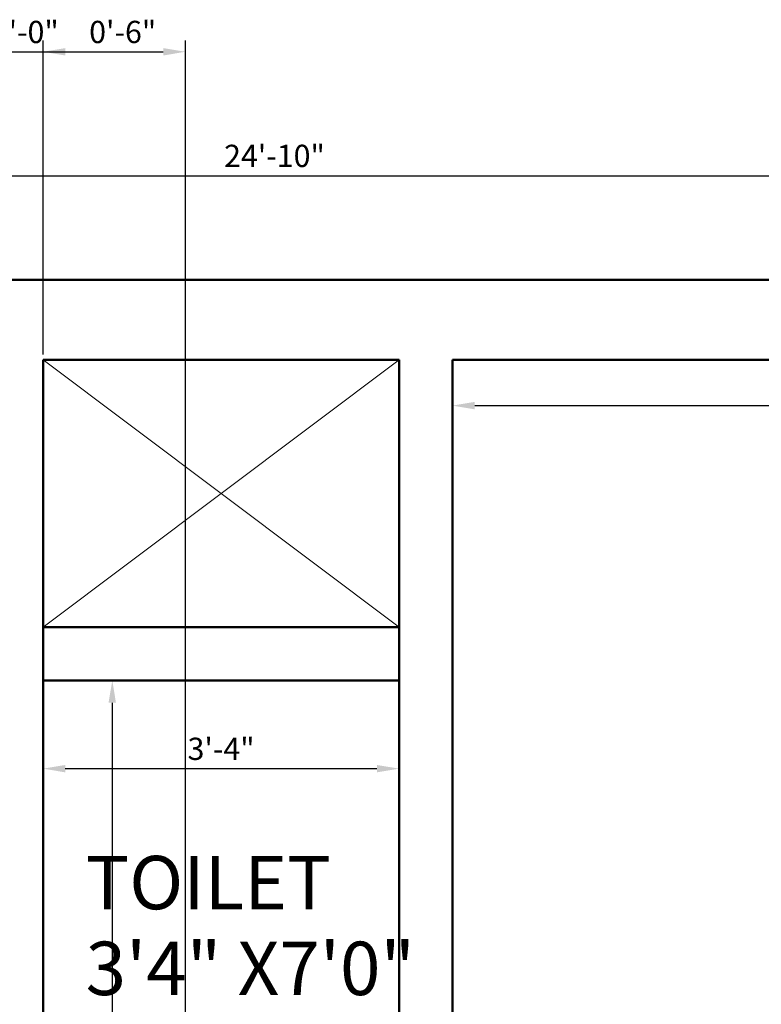
# Model space of a CAD drawing. Units: inches. Extents: x 2385 to 2740, y 1752 to 2305.
# Tile 13 of 15: x 2535 to 2618, y 2195 to 2305. Entities that reach past the tile are written whole.
import ezdxf

# ---------------------------------------------------------------- set-up
doc = ezdxf.new("R2010")
doc.units = ezdxf.units.IN
for name, color, linetype, lineweight in [('A-ANNO-DIMS', 2, 'Continuous', 18), ('A-AREA-IDEN', 7, 'Continuous', 25), ('A-FLOR-OPEN', 8, 'Continuous', 18), ('A-WALL', 7, 'Continuous', 50)]:
    doc.layers.add(name, color=color, linetype=linetype, lineweight=lineweight)
doc.styles.get("Standard").update_dxf_attribs({"font": 'arial.ttf'})
doc.dimstyles.new('Copy of ISO-25', dxfattribs={"dimtxt": 2.5, "dimasz": 2.5, "dimexe": 1.25, "dimexo": 0.625, "dimtad": 1, "dimdec": 1, "dimlunit": 4, "dimtxsty": 'Standard', "dimcen": 2.5, "dimadec": 0, "dimazin": 0, "dimtfac": 1, "dimtdec": 1, "dimtmove": 0, "dimatfit": 3, "dimfxl": 1, "dimarcsym": 0})

# ---------------------------------------------------------------- blocks, each defined once
blk = doc.blocks.new('*D8')
at = {"layer": 'A-ANNO-DIMS', "color": 0, "lineweight": -2, "transparency": 16777216}
for p, q in [((2583.25, 2266.34), (2583.25, 2260.59)), ((2703.25, 2266.34), (2703.25, 2260.59)), ((2585.75, 2261.84), (2700.75, 2261.84))]:
    blk.add_line(p, q, dxfattribs=at)
at = {"layer": 'A-ANNO-DIMS', "color": 0, "transparency": 16777216}
for points in [[(2585.75, 2262.26), (2585.75, 2261.42), (2583.25, 2261.84)], [(2700.75, 2262.26), (2700.75, 2261.42), (2703.25, 2261.84)]]:
    blk.add_solid(points, dxfattribs=at)
at = {"layer": 'Defpoints', "color": 0, "transparency": 16777216}
for p in [(2583.25, 2266.97), (2703.25, 2266.97), (2703.25, 2261.84)]:
    blk.add_point(p, dxfattribs=at)
at = {"layer": 'A-ANNO-DIMS', "color": 0, "transparency": 16777216, "insert": (2643.25, 2263.74), "char_height": 2.5, "attachment_point": 5}
blk.add_mtext("10'", dxfattribs=at)
blk = doc.blocks.new('*D10')
at = {"layer": 'A-ANNO-DIMS', "color": 0, "lineweight": -2, "transparency": 16777216}
for p, q in [((2537.25, 2230.34), (2537.25, 2219.81)), ((2577.25, 2230.34), (2577.25, 2219.81)), ((2539.75, 2221.06), (2574.75, 2221.06))]:
    blk.add_line(p, q, dxfattribs=at)
at = {"layer": 'A-ANNO-DIMS', "color": 0, "transparency": 16777216}
for points in [[(2539.75, 2221.47), (2539.75, 2220.64), (2537.25, 2221.06)], [(2574.75, 2221.47), (2574.75, 2220.64), (2577.25, 2221.06)]]:
    blk.add_solid(points, dxfattribs=at)
at = {"layer": 'Defpoints', "color": 0, "transparency": 16777216}
for p in [(2537.25, 2230.97), (2577.25, 2230.97), (2577.25, 2221.06)]:
    blk.add_point(p, dxfattribs=at)
at = {"layer": 'A-ANNO-DIMS', "color": 0, "transparency": 16777216, "insert": (2557.25, 2222.96), "char_height": 2.5, "attachment_point": 5}
blk.add_mtext('3\'-4"', dxfattribs=at)
blk = doc.blocks.new('*D11')
at = {"layer": 'A-ANNO-DIMS', "color": 0, "lineweight": -2, "transparency": 16777216}
for p, q in [((2537.87, 2230.97), (2546.28, 2230.97)), ((2545.03, 2228.47), (2545.03, 2149.47)), ((2537.87, 2146.97), (2546.28, 2146.97))]:
    blk.add_line(p, q, dxfattribs=at)
at = {"layer": 'A-ANNO-DIMS', "color": 0, "transparency": 16777216}
for points in [[(2544.61, 2228.47), (2545.44, 2228.47), (2545.03, 2230.97)], [(2544.61, 2149.47), (2545.44, 2149.47), (2545.03, 2146.97)]]:
    blk.add_solid(points, dxfattribs=at)
at = {"layer": 'Defpoints', "color": 0, "transparency": 16777216}
for p in [(2537.25, 2230.97), (2537.25, 2146.97), (2545.03, 2146.97)]:
    blk.add_point(p, dxfattribs=at)
at = {"layer": 'A-ANNO-DIMS', "color": 0, "transparency": 16777216, "insert": (2543.15, 2188.97), "char_height": 2.5, "attachment_point": 5, "rotation": 90}
blk.add_mtext("7'", dxfattribs=at)
blk = doc.blocks.new('*D24')
at = {"layer": 'A-ANNO-DIMS', "color": 0, "lineweight": -2, "transparency": 16777216}
for p, q in [((2414.25, 2276.59), (2414.25, 2288.91)), ((2712.25, 2276.59), (2712.25, 2288.91)), ((2416.75, 2287.66), (2709.75, 2287.66))]:
    blk.add_line(p, q, dxfattribs=at)
at = {"layer": 'A-ANNO-DIMS', "color": 0, "transparency": 16777216}
for points in [[(2416.75, 2288.08), (2416.75, 2287.25), (2414.25, 2287.66)], [(2709.75, 2288.08), (2709.75, 2287.25), (2712.25, 2287.66)]]:
    blk.add_solid(points, dxfattribs=at)
at = {"layer": 'Defpoints', "color": 0, "transparency": 16777216}
for p in [(2712.25, 2287.66), (2414.25, 2275.97), (2712.25, 2275.97)]:
    blk.add_point(p, dxfattribs=at)
at = {"layer": 'A-ANNO-DIMS', "color": 0, "transparency": 16777216, "insert": (2563.25, 2289.57), "char_height": 2.5, "attachment_point": 5}
blk.add_mtext('24\'-10"', dxfattribs=at)
blk = doc.blocks.new('*D39')
at = {"layer": 'A-ANNO-DIMS', "color": 0, "lineweight": -2, "transparency": 16777216}
for p, q in [((2531.25, 2267.59), (2531.25, 2302.84)), ((2537.25, 2267.59), (2537.25, 2302.84)), ((2528.75, 2301.59), (2526.25, 2301.59)), ((2531.25, 2301.59), (2537.25, 2301.59)), ((2539.75, 2301.59), (2550.14, 2301.59))]:
    blk.add_line(p, q, dxfattribs=at)
at = {"layer": 'A-ANNO-DIMS', "color": 0, "transparency": 16777216}
for points in [[(2528.75, 2302), (2528.75, 2301.17), (2531.25, 2301.59)], [(2539.75, 2302), (2539.75, 2301.17), (2537.25, 2301.59)]]:
    blk.add_solid(points, dxfattribs=at)
at = {"layer": 'Defpoints', "color": 0, "transparency": 16777216}
for p in [(2537.25, 2301.59), (2531.25, 2266.97), (2537.25, 2266.97)]:
    blk.add_point(p, dxfattribs=at)
at = {"layer": 'A-ANNO-DIMS', "color": 0, "transparency": 16777216, "insert": (2546.2, 2303.49), "char_height": 2.5, "attachment_point": 5}
blk.add_mtext('0\'-6"', dxfattribs=at)
blk = doc.blocks.new('*D48')
at = {"layer": 'A-ANNO-DIMS', "color": 0, "lineweight": -2, "transparency": 16777216}
for p, q in [((2517.25, 1916.59), (2517.25, 2302.84)), ((2553.25, 1916.59), (2553.25, 2302.84)), ((2519.75, 2301.59), (2550.75, 2301.59))]:
    blk.add_line(p, q, dxfattribs=at)
at = {"layer": 'A-ANNO-DIMS', "color": 0, "transparency": 16777216}
for points in [[(2519.75, 2302), (2519.75, 2301.17), (2517.25, 2301.59)], [(2550.75, 2302), (2550.75, 2301.17), (2553.25, 2301.59)]]:
    blk.add_solid(points, dxfattribs=at)
at = {"layer": 'Defpoints', "color": 0, "transparency": 16777216}
for p in [(2553.25, 2301.59), (2517.25, 1915.97), (2553.25, 1915.97)]:
    blk.add_point(p, dxfattribs=at)
at = {"layer": 'A-ANNO-DIMS', "color": 0, "transparency": 16777216, "insert": (2535.25, 2303.49), "char_height": 2.5, "attachment_point": 5}
blk.add_mtext('3\'-0"', dxfattribs=at)

msp = doc.modelspace()

# ---------------------------------------------------------------- linework, layer by layer
at = {"layer": 'A-FLOR-OPEN'}
for p, q in [((2537.25, 2266.97), (2577.25, 2236.97)), ((2577.25, 2266.97), (2537.25, 2236.97))]:
    msp.add_line(p, q, dxfattribs=at)
at = {"layer": 'A-WALL'}
for p, q in [((2414.25, 2275.97), (2694.25, 2275.97)), ((2414.25, 2275.97), (2712.25, 2275.97)), ((2583.25, 2275.97), (2577.25, 2275.97)), ((2577.25, 2266.97), (2537.25, 2266.97)), ((2577.25, 2266.97), (2537.25, 2266.97)), ((2537.25, 2266.97), (2537.25, 2146.97)), ((2577.25, 2266.97), (2577.25, 2182.97)), ((2583.25, 2182.97), (2583.25, 2266.97)), ((2703.25, 2266.97), (2583.25, 2266.97)), ((2577.25, 2236.97), (2537.25, 2236.97)), ((2577.25, 2230.97), (2577.25, 2236.97)), ((2537.25, 2146.97), (2537.25, 2230.97)), ((2537.25, 2230.97), (2577.25, 2230.97))]:
    msp.add_line(p, q, dxfattribs=at)

# ---------------------------------------------------------------- texts
at = {"layer": 'A-AREA-IDEN'}
for s, p in [('TOILET', (2542.03, 2205.26)), ('3\'4" X7\'0"', (2542.03, 2195.62))]:
    msp.add_text(s, height=6, dxfattribs=at).set_placement(p)

# ---------------------------------------------------------------- dimensions: what is measured, and where the dimension line sits
at = {"layer": 'A-ANNO-DIMS'}
for base, p1, p2, override, picture, middle in [((2553.25, 2301.59), (2517.25, 1915.97), (2553.25, 1915.97), {"dimdec": 1, "dimlfac": 1, "dimrnd": 0, "dimzin": 1, "dimdsep": 46, "dimlunit": 4, "dimfrac": 2}, '*D48', (2535.25, 2303.49)), ((2537.25, 2301.59), (2531.25, 2266.97), (2537.25, 2266.97), {"dimdec": 1, "dimlfac": 1, "dimrnd": 0, "dimzin": 1, "dimdsep": 46, "dimlunit": 4, "dimfrac": 2}, '*D39', (2546.2, 2303.49)), ((2712.25, 2287.66), (2414.25, 2275.97), (2712.25, 2275.97), {"dimclrd": 0, "dimclre": 0, "dimclrt": 0}, '*D24', (2563.25, 2289.57)), ((2703.25, 2261.84), (2583.25, 2266.97), (2703.25, 2266.97), {"dimclrd": 0, "dimclre": 0, "dimclrt": 0}, '*D8', (2643.25, 2263.74)), ((2577.25, 2221.06), (2537.25, 2230.97), (2577.25, 2230.97), {"dimclrd": 0, "dimclre": 0, "dimclrt": 0}, '*D10', (2557.25, 2222.96))]:
    dim = msp.add_linear_dim(base=base, p1=p1, p2=p2, dimstyle='Copy of ISO-25', override=override, dxfattribs=at)
    dim.commit()
    dim.dimension.update_dxf_attribs({"geometry": picture, "text_midpoint": middle})
dim = msp.add_linear_dim(base=(2545.03, 2146.97), p1=(2537.25, 2230.97), p2=(2537.25, 2146.97), angle=90, dimstyle='Copy of ISO-25', override={"dimclrd": 0, "dimclre": 0, "dimclrt": 0}, dxfattribs=at)
dim.commit()
dim.dimension.update_dxf_attribs({"geometry": '*D11', "text_midpoint": (2543.15, 2188.97)})

doc.saveas('drawing.dxf')
